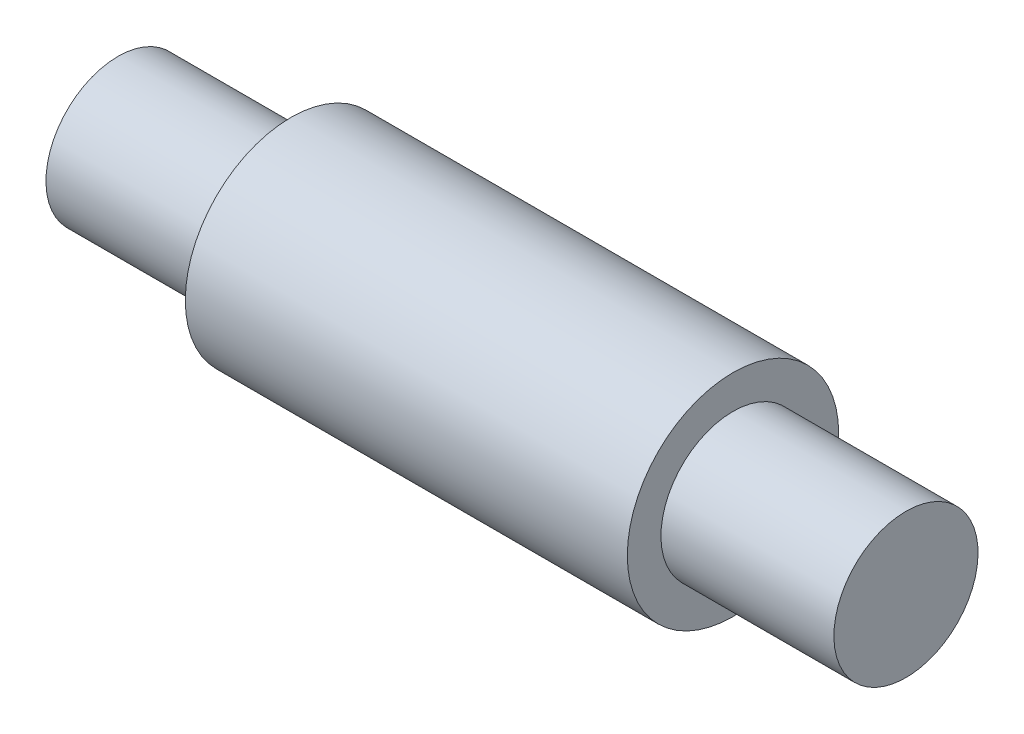
SolidWorks part; units mm, degrees
material "Plain Carbon Steel"
ref_plane "Front Plane" through (0, 0, 0) normal (0, 0, 1) x (1, 0, 0)
ref_plane "Top Plane" through (0, 0, 0) normal (0, 1, 0) x (1, 0, 0)
ref_plane "Right Plane" through (0, 0, 0) normal (1, 0, 0) x (0, 0, -1)
sketch "Spacer Profile Sketch" plane through (0, 0, 0) normal (0, 0, 1) x (1, 0, 0)
  line L0 (0, 0) -> (-82, 0) construction
  line L1 (-82, 0) -> (-82, 7.5)
  line L2 (-82, 7.5) -> (-64, 7.5)
  line L3 (-64, 7.5) -> (-64, 11)
  line L4 (-64, 11) -> (-18, 11)
  line L5 (-18, 11) -> (-18, 7.5)
  line L6 (-18, 7.5) -> (0, 7.5)
  line L7 (0, 7.5) -> (0, 0)
  line L8 (0, 0) -> (-82, 0)
  dimension "D1" = 11
  dimension "D2" = 82
  dimension "D3" = 18
  dimension "D4" = 18
  dimension "D5" = 7.5
  dimension "D6" = 7.5
revolve "Spacer Body Revolve" add sketch "Spacer Profile Sketch" angle 360 about L0
cosmetic thread "Cosmetic Thread1"
cosmetic thread "Cosmetic Thread2"
